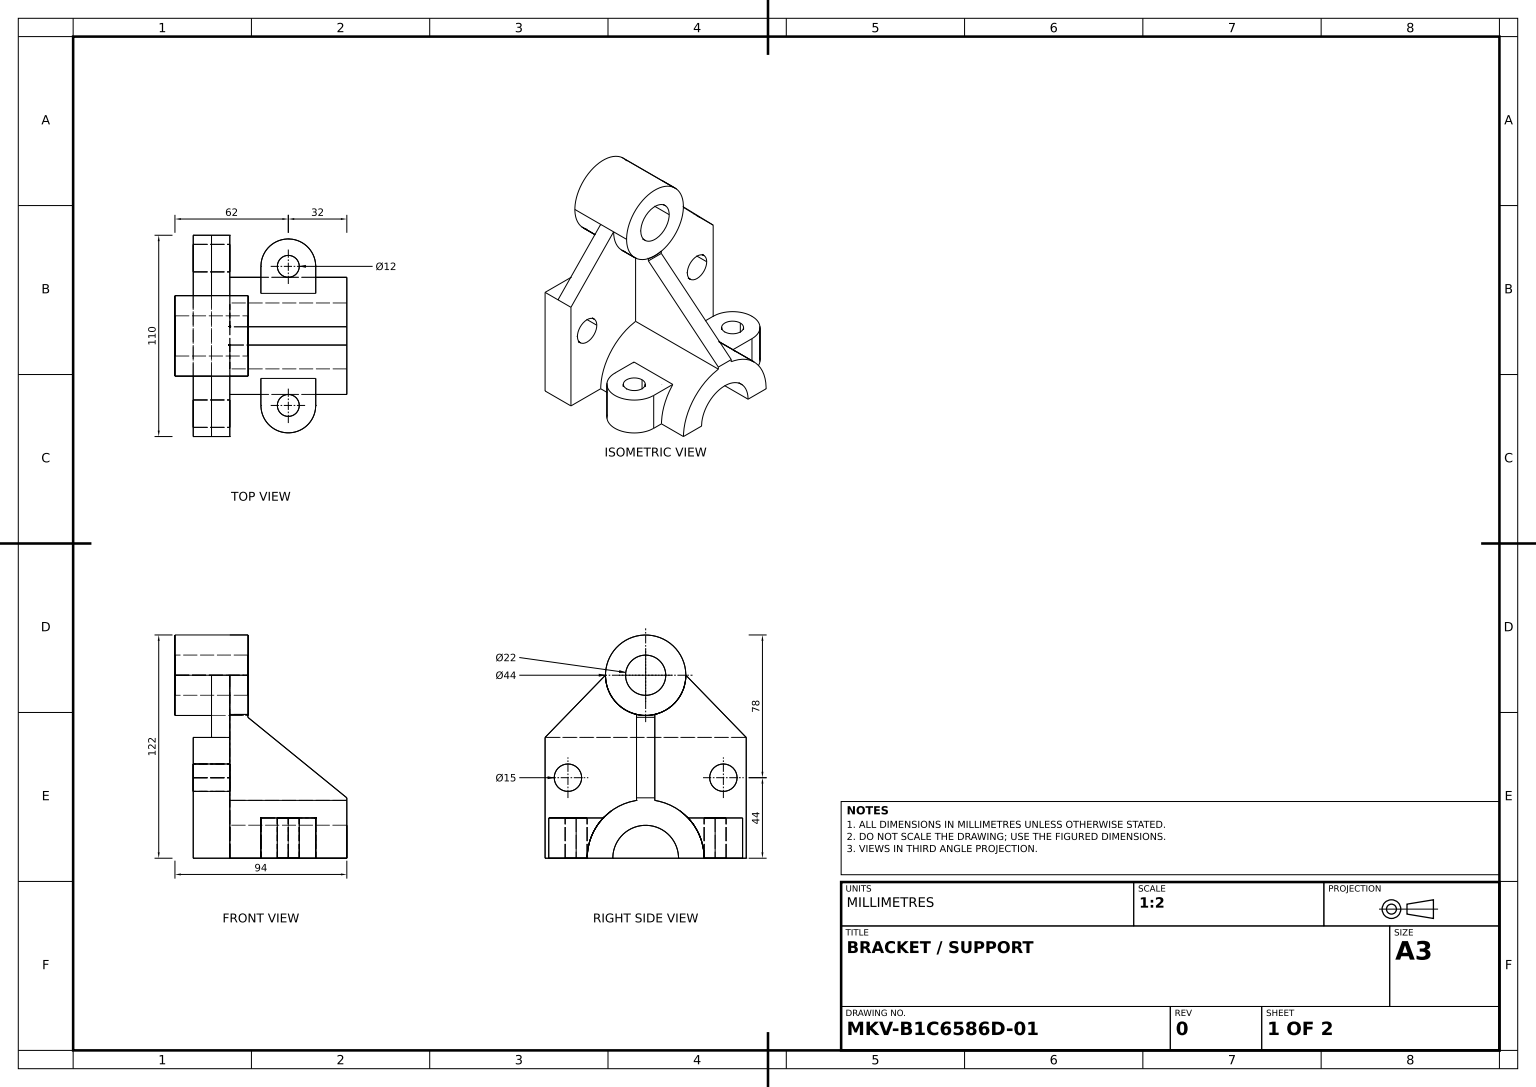
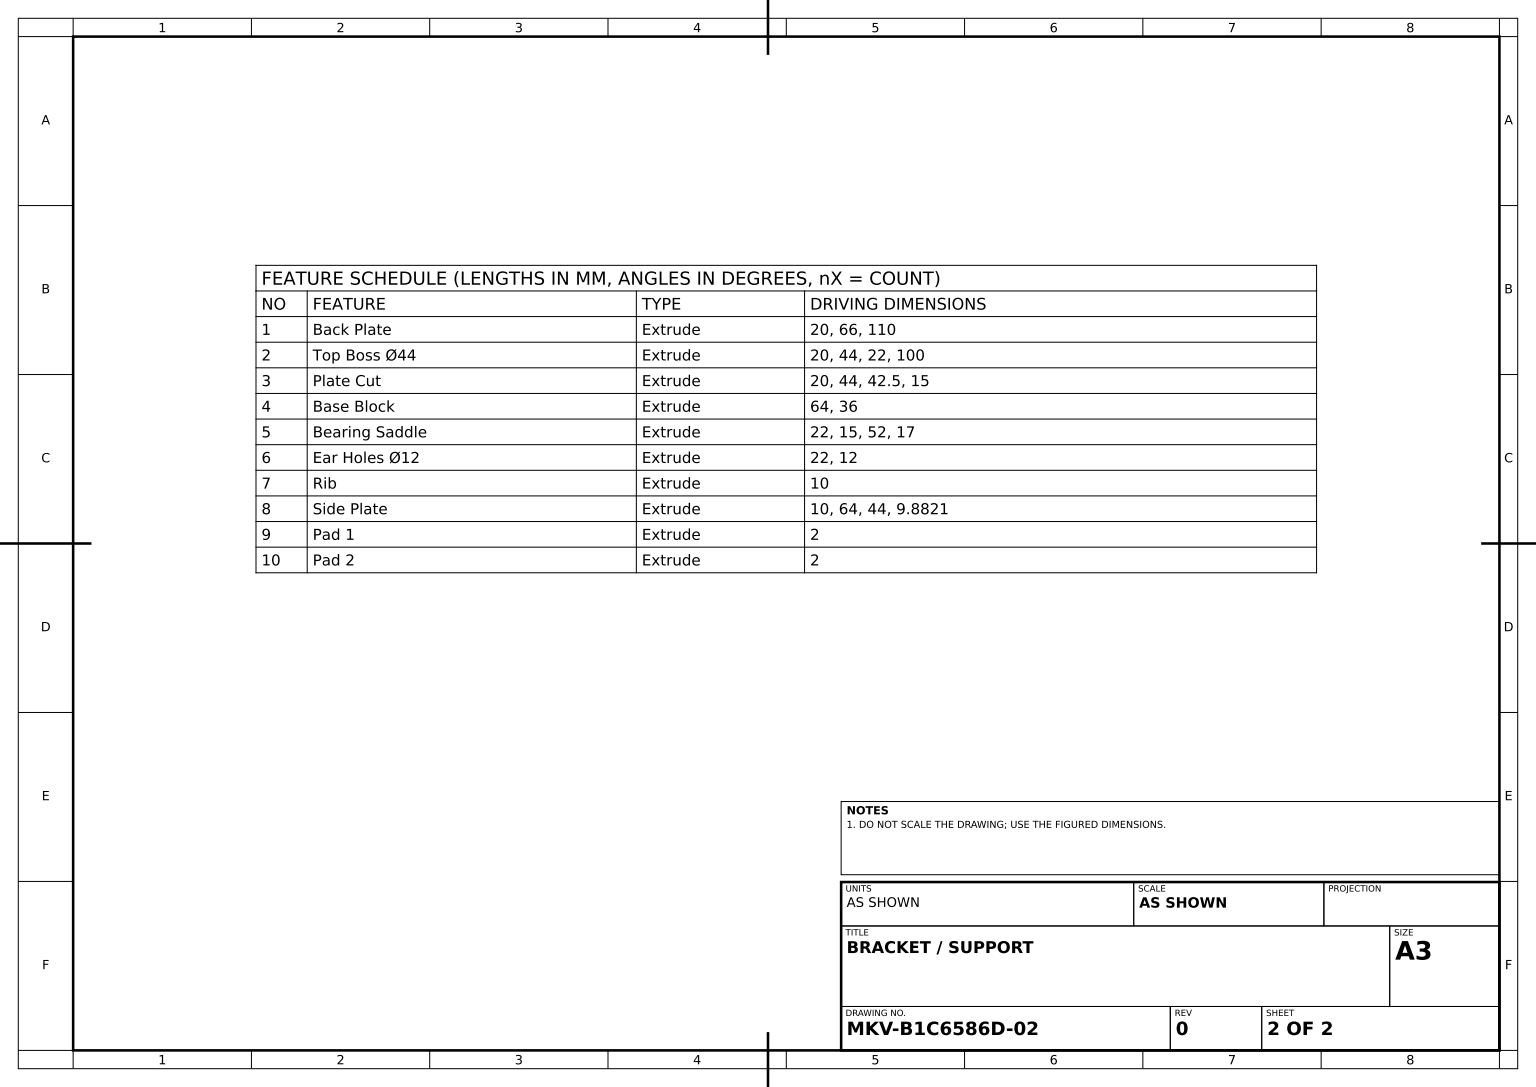
from build123d import *

# Parameters (mm, degrees)
BACK_PLATE_SKETCH_W    = 110
BACK_PLATE_SKETCH_H    = 66
BACK_PLATE_DEPTH       = 10
TOP_BOSS_44_DEPTH      = 20
TOP_BOSS_44_DEPTH_BACK = 20
TOP_BOSS_SKETCH_R      = 22
TOP_BOSS_SKETCH_R_2    = 11
PLATE_CUT_SKETCH_R     = 7.5
PLATE_CUT_DEPTH        = 20
BASE_BLOCK_DEPTH       = 64
BEARING_SADDLE_DEPTH   = 22
EAR_HOLES_SKETCH_R     = 6
EAR_HOLES_12_DEPTH     = 22
RIB_DEPTH              = 10
SIDE_PLATE_DEPTH       = 5
PAD_1_SKETCH_W         = 9.88210357
PAD_1_SKETCH_H         = 10
PAD_1_DEPTH            = 2
PAD_2_SKETCH_W         = 64
PAD_2_SKETCH_H         = 10
PAD_2_DEPTH            = 2


with BuildPart() as part:
    # Back Plate Sketch → Back Plate (new, symmetric)
    with BuildSketch(Plane(origin=(0, 0, 0), x_dir=(0, 0, -1), z_dir=(1, 0, 0))):
        Rectangle(BACK_PLATE_SKETCH_W, BACK_PLATE_SKETCH_H)
    extrude(amount=BACK_PLATE_DEPTH, both=True)

    # Plate Cut Sketch → Plate Cut (cut)
    with BuildSketch(Plane(origin=(10, 0, 0), x_dir=(0, 0, -1), z_dir=(1, 0, 0))):
        with Locations((42.5, 11)):
            Circle(PLATE_CUT_SKETCH_R)
        with Locations(Location((-42.5, 11, 0), (0, 0, 180))):
            Circle(PLATE_CUT_SKETCH_R)
    extrude(amount=-PLATE_CUT_DEPTH, mode=Mode.SUBTRACT)

    # Base Block Sketch → Base Block (add)
    with BuildSketch(Plane(origin=(10, 0, 0), x_dir=(0, 0, -1), z_dir=(1, 0, 0))):
        with BuildLine():
            Line((-32, -33), (-18, -33))
            ThreePointArc((-18, -33), (0, -15), (18, -33))
            Line((18, -33), (32, -33))
            ThreePointArc((32, -33), (0, -1), (-32, -33))
        make_face()
    extrude(amount=BASE_BLOCK_DEPTH)

    # Bearing Saddle Sketch → Bearing Saddle (add)
    with BuildSketch(Plane.XZ.offset(33)):
        with BuildLine():
            Line((27, 38), (27, 18))
            Line((27, 18), (57, 18))
            Line((57, 18), (57, 38))
            ThreePointArc((57, 38), (42, 53), (27, 38))
        make_face()
        with BuildLine():
            Line((27, -38), (27, -18))
            Line((27, -18), (57, -18))
            Line((57, -18), (57, -38))
            ThreePointArc((57, -38), (42, -53), (27, -38))
        make_face()
    extrude(amount=-BEARING_SADDLE_DEPTH)

    # Ear Holes Sketch → Ear Holes Ø12 (cut)
    with BuildSketch(Plane(origin=(0, -11, 0), x_dir=(1, 0, 0), z_dir=(0, 1, 0))):
        with Locations(Location((42, 38, 0), (0, 0, 270))):
            Circle(EAR_HOLES_SKETCH_R)
        with Locations(Location((42, -38, 0), (0, 0, 270))):
            Circle(EAR_HOLES_SKETCH_R)
    extrude(amount=-EAR_HOLES_12_DEPTH, mode=Mode.SUBTRACT)



with BuildPart() as body_2:
    # Top Boss Sketch → Top Boss Ø44 (new, two sides: drawn at the far end of the back side and taken through both)
    with BuildSketch(Plane(origin=(0, 0, 0), x_dir=(0, 0, -1), z_dir=(1, 0, 0)).offset(-TOP_BOSS_44_DEPTH_BACK)):
        with Locations((0, 67)):
            Circle(TOP_BOSS_SKETCH_R)
        with Locations((0, 67)):
            Circle(TOP_BOSS_SKETCH_R_2, mode=Mode.SUBTRACT)
    extrude(amount=TOP_BOSS_44_DEPTH + TOP_BOSS_44_DEPTH_BACK)


with BuildPart() as part_1:
    add(part.part)

    add(body_2.part)  # Rib merges body 2
    # Rib Sketch → Rib (add)
    with BuildSketch(Plane(origin=(10, 0, 0), x_dir=(0, 0, -1), z_dir=(1, 0, 0))):
        with BuildLine():
            Line((-22, 67), (-55, 33))
            Line((-55, 33), (55, 33))
            Line((55, 33), (22, 67))
            ThreePointArc((22, 67), (0, 45), (-22, 67))
        make_face()
    extrude(amount=-RIB_DEPTH)

    # Side Plate Sketch → Side Plate (add, symmetric)
    with BuildSketch(Plane.XY):
        Polygon((10, 44), (19.88210357, 44), (74, 0), (10, 0), align=None)
    extrude(amount=SIDE_PLATE_DEPTH, both=True)

    # Pad 1 Sketch → Pad 1 (add)
    with BuildSketch(Plane(origin=(0, 44, 0), x_dir=(1, 0, 0), z_dir=(0, 1, 0))):
        with Locations((14.941051785, 0)):
            Rectangle(PAD_1_SKETCH_W, PAD_1_SKETCH_H)
    extrude(amount=PAD_1_DEPTH)

    # Pad 2 Sketch → Pad 2 (add)
    with BuildSketch(Plane.XZ):
        with Locations((42, 0)):
            Rectangle(PAD_2_SKETCH_W, PAD_2_SKETCH_H)
    extrude(amount=PAD_2_DEPTH)


solid = part_1.part
